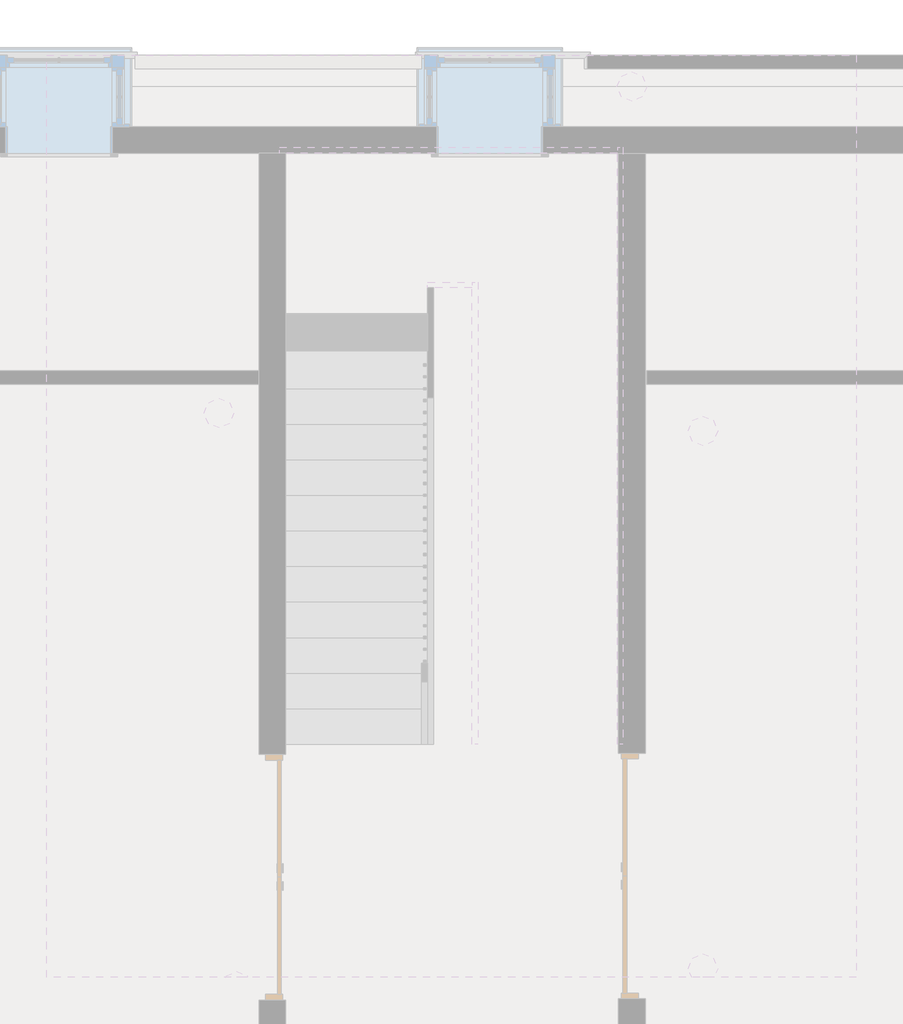
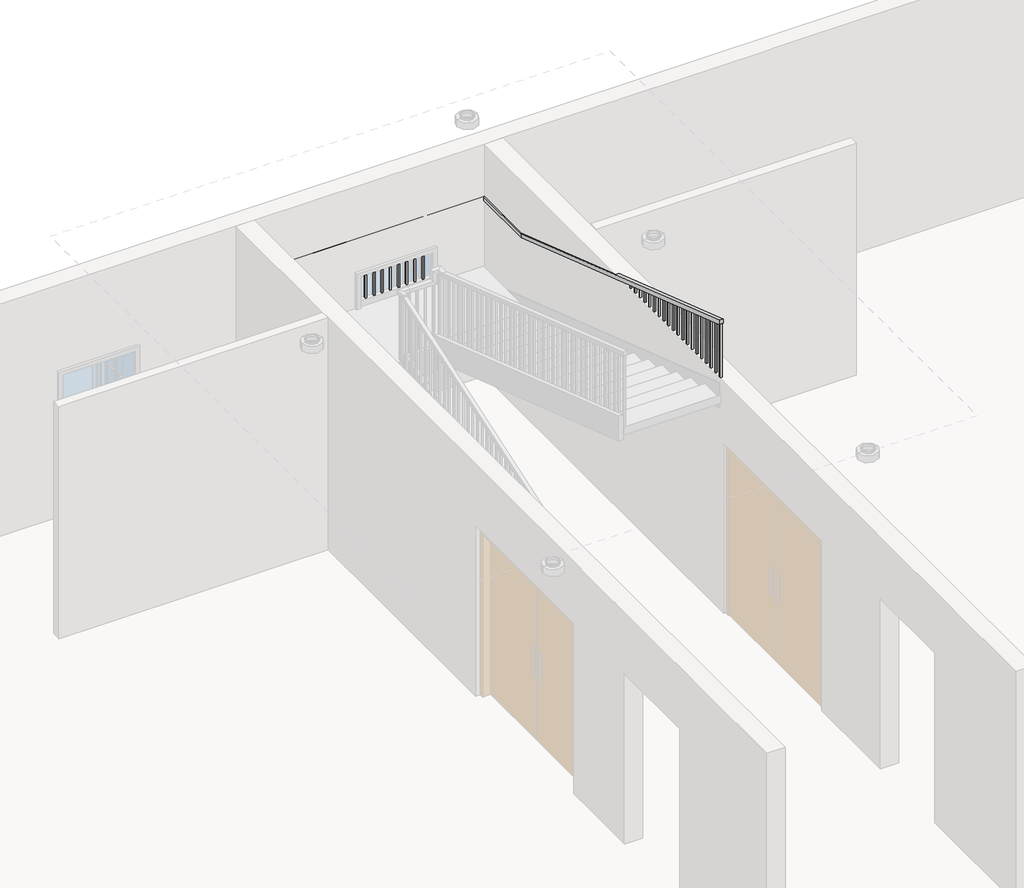
# One storey, part 5 of 7: 1 railing.
"""IFC4 building model written with IfcOpenShell, lengths in millimetres."""

from ifc_helpers import new_model, si_unit, frame, origin, place, context, project, spatial, polyline, outline, extrude, faceted_brep, element, save

model = new_model("IFC4")

# Units and contexts
model_context = context("Model", 3, world=origin())
ifc_project = project(units=[si_unit("LENGTHUNIT", "METRE", prefix="MILLI")], contexts=[model_context])

# Site, building, storey
site = spatial("IfcSite", under=ifc_project)
building = spatial("IfcBuilding", under=site)
storey = spatial("IfcBuildingStorey", under=building, Elevation=3200.4)

# Railing
placement = place(None, origin())
element("IfcRailing", 1, ObjectType="Handrail - Rectangular", at=placement, inside=storey, context=model_context, shape_type="SolidModel", body=[
    faceted_brep([(-1899.5987998, 2564.5067329, 4218.2142857), (-1899.5987998, 2564.5067329, 4164.5699957), (-1848.7987998, 2564.5067329, 4164.5699957), (-1848.7987998, 2564.5067329, 4218.2142857), (-1899.5987998, 6526.9067329, 5562.6), (-1899.5987998, 6535.2899033, 5511.8), (-1848.7987998, 6535.2899033, 5511.8), (-1848.7987998, 6526.9067329, 5562.6), (-1899.5987998, 7682.6067329, 5511.8), (-1899.5987998, 7682.6067329, 5562.6), (1046.8012002, 7682.6067329, 5562.6), (1046.8012002, 7682.6067329, 5511.8), (-1848.7987998, 7631.8067329, 5511.8), (996.0012002, 7631.8067329, 5511.8), (-1848.7987998, 7631.8067329, 5562.6), (996.0012002, 7631.8067329, 5562.6), (1046.8012002, 6831.7067329, 5562.6), (1046.8012002, 6823.3235624, 5511.8), (996.0012002, 6823.3235624, 5511.8), (996.0012002, 6831.7067329, 5562.6), (1046.8012002, 2564.5067329, 7010.4), (996.0012002, 2564.5067329, 7010.4), (996.0012002, 2564.5067329, 6956.75571), (1046.8012002, 2564.5067329, 6956.75571)], [[[0, 1, 2, 3]], [[1, 0, 4, 5]], [[2, 1, 5, 6]], [[3, 2, 6, 7]], [[0, 3, 7, 4]], [[8, 9, 10, 11]], [[12, 8, 11, 13]], [[14, 12, 13, 15]], [[9, 14, 15, 10]], [[11, 10, 16, 17]], [[13, 11, 17, 18]], [[15, 13, 18, 19]], [[10, 15, 19, 16]], [[5, 4, 9, 8]], [[6, 5, 8, 12]], [[7, 6, 12, 14]], [[4, 7, 14, 9]], [[20, 21, 22, 23]], [[17, 16, 20, 23]], [[18, 17, 23, 22]], [[19, 18, 22, 21]], [[16, 19, 21, 20]]]),
    extrude(outline(polyline([(2586.7317329, 6949.215085), (2586.7317329, 6178.2831452), (2567.6817329, 6184.7465381), (2567.6817329, 6955.6784779), (2586.7317329, 6949.215085)])), frame((1011.8762002, 0.0, 0.0), z_axis=(1.0, 0.0, 0.0), x_axis=(0.0, 1.0, 0.0)), (0.0, 0.0, 1.0), 19.05),
    extrude(outline(polyline([(2688.3317329, 6914.7436565), (2688.3317329, 6143.8117167), (2669.2817329, 6150.2751095), (2669.2817329, 6921.2070493), (2688.3317329, 6914.7436565)])), frame((1011.8762002, 0.0, 0.0), z_axis=(1.0, 0.0, 0.0), x_axis=(0.0, 1.0, 0.0)), (0.0, 0.0, 1.0), 19.05),
    extrude(outline(polyline([(2789.9317329, 6880.2722279), (2789.9317329, 6109.3402881), (2770.8817329, 6115.803681), (2770.8817329, 6886.7356207), (2789.9317329, 6880.2722279)])), frame((1011.8762002, 0.0, 0.0), z_axis=(1.0, 0.0, 0.0), x_axis=(0.0, 1.0, 0.0)), (0.0, 0.0, 1.0), 19.05),
    extrude(outline(polyline([(2891.5317329, 6845.8007993), (2891.5317329, 6074.8688595), (2872.4817329, 6081.3322524), (2872.4817329, 6852.2641922), (2891.5317329, 6845.8007993)])), frame((1011.8762002, 0.0, 0.0), z_axis=(1.0, 0.0, 0.0), x_axis=(0.0, 1.0, 0.0)), (0.0, 0.0, 1.0), 19.05),
    extrude(outline(polyline([(2993.1317329, 6811.3293707), (2993.1317329, 6040.397431), (2974.0817329, 6046.8608238), (2974.0817329, 6817.7927636), (2993.1317329, 6811.3293707)])), frame((1011.8762002, 0.0, 0.0), z_axis=(1.0, 0.0, 0.0), x_axis=(0.0, 1.0, 0.0)), (0.0, 0.0, 1.0), 19.05),
    extrude(outline(polyline([(3094.7317329, 6776.8579422), (3094.7317329, 6005.9260024), (3075.6817329, 6012.3893952), (3075.6817329, 6783.321335), (3094.7317329, 6776.8579422)])), frame((1011.8762002, 0.0, 0.0), z_axis=(1.0, 0.0, 0.0), x_axis=(0.0, 1.0, 0.0)), (0.0, 0.0, 1.0), 19.05),
    extrude(outline(polyline([(3196.3317329, 6742.3865136), (3196.3317329, 5971.4545738), (3177.2817329, 5977.9179667), (3177.2817329, 6748.8499065), (3196.3317329, 6742.3865136)])), frame((1011.8762002, 0.0, 0.0), z_axis=(1.0, 0.0, 0.0), x_axis=(0.0, 1.0, 0.0)), (0.0, 0.0, 1.0), 19.05),
    extrude(outline(polyline([(3297.9317329, 6707.915085), (3297.9317329, 5936.9831452), (3278.8817329, 5943.4465381), (3278.8817329, 6714.3784779), (3297.9317329, 6707.915085)])), frame((1011.8762002, 0.0, 0.0), z_axis=(1.0, 0.0, 0.0), x_axis=(0.0, 1.0, 0.0)), (0.0, 0.0, 1.0), 19.05),
    extrude(outline(polyline([(3399.5317329, 6673.4436565), (3399.5317329, 5902.5117167), (3380.4817329, 5908.9751095), (3380.4817329, 6679.9070493), (3399.5317329, 6673.4436565)])), frame((1011.8762002, 0.0, 0.0), z_axis=(1.0, 0.0, 0.0), x_axis=(0.0, 1.0, 0.0)), (0.0, 0.0, 1.0), 19.05),
    extrude(outline(polyline([(3501.1317329, 6638.9722279), (3501.1317329, 5868.0402881), (3482.0817329, 5874.503681), (3482.0817329, 6645.4356207), (3501.1317329, 6638.9722279)])), frame((1011.8762002, 0.0, 0.0), z_axis=(1.0, 0.0, 0.0), x_axis=(0.0, 1.0, 0.0)), (0.0, 0.0, 1.0), 19.05),
    extrude(outline(polyline([(3602.7317329, 6604.5007993), (3602.7317329, 5833.5688595), (3583.6817329, 5840.0322524), (3583.6817329, 6610.9641922), (3602.7317329, 6604.5007993)])), frame((1011.8762002, 0.0, 0.0), z_axis=(1.0, 0.0, 0.0), x_axis=(0.0, 1.0, 0.0)), (0.0, 0.0, 1.0), 19.05),
    extrude(outline(polyline([(3704.3317329, 6570.0293707), (3704.3317329, 5799.097431), (3685.2817329, 5805.5608238), (3685.2817329, 6576.4927636), (3704.3317329, 6570.0293707)])), frame((1011.8762002, 0.0, 0.0), z_axis=(1.0, 0.0, 0.0), x_axis=(0.0, 1.0, 0.0)), (0.0, 0.0, 1.0), 19.05),
    extrude(outline(polyline([(3805.9317329, 6535.5579422), (3805.9317329, 5764.6260024), (3786.8817329, 5771.0893952), (3786.8817329, 6542.021335), (3805.9317329, 6535.5579422)])), frame((1011.8762002, 0.0, 0.0), z_axis=(1.0, 0.0, 0.0), x_axis=(0.0, 1.0, 0.0)), (0.0, 0.0, 1.0), 19.05),
    extrude(outline(polyline([(3907.5317329, 6501.0865136), (3907.5317329, 5730.1545738), (3888.4817329, 5736.6179667), (3888.4817329, 6507.5499065), (3907.5317329, 6501.0865136)])), frame((1011.8762002, 0.0, 0.0), z_axis=(1.0, 0.0, 0.0), x_axis=(0.0, 1.0, 0.0)), (0.0, 0.0, 1.0), 19.05),
    extrude(outline(polyline([(4009.1317329, 6466.615085), (4009.1317329, 5695.6831452), (3990.0817329, 5702.1465381), (3990.0817329, 6473.0784779), (4009.1317329, 6466.615085)])), frame((1011.8762002, 0.0, 0.0), z_axis=(1.0, 0.0, 0.0), x_axis=(0.0, 1.0, 0.0)), (0.0, 0.0, 1.0), 19.05),
    extrude(outline(polyline([(4110.7317329, 6432.1436565), (4110.7317329, 5661.2117167), (4091.6817329, 5667.6751095), (4091.6817329, 6438.6070493), (4110.7317329, 6432.1436565)])), frame((1011.8762002, 0.0, 0.0), z_axis=(1.0, 0.0, 0.0), x_axis=(0.0, 1.0, 0.0)), (0.0, 0.0, 1.0), 19.05),
    extrude(outline(polyline([(4212.3317329, 6397.6722279), (4212.3317329, 5626.7402881), (4193.2817329, 5633.203681), (4193.2817329, 6404.1356207), (4212.3317329, 6397.6722279)])), frame((1011.8762002, 0.0, 0.0), z_axis=(1.0, 0.0, 0.0), x_axis=(0.0, 1.0, 0.0)), (0.0, 0.0, 1.0), 19.05),
    extrude(outline(polyline([(4313.9317329, 6363.2007993), (4313.9317329, 5592.2688595), (4294.8817329, 5598.7322524), (4294.8817329, 6369.6641922), (4313.9317329, 6363.2007993)])), frame((1011.8762002, 0.0, 0.0), z_axis=(1.0, 0.0, 0.0), x_axis=(0.0, 1.0, 0.0)), (0.0, 0.0, 1.0), 19.05),
    extrude(outline(polyline([(4415.5317329, 6328.7293707), (4415.5317329, 5557.797431), (4396.4817329, 5564.2608238), (4396.4817329, 6335.1927636), (4415.5317329, 6328.7293707)])), frame((1011.8762002, 0.0, 0.0), z_axis=(1.0, 0.0, 0.0), x_axis=(0.0, 1.0, 0.0)), (0.0, 0.0, 1.0), 19.05),
    extrude(outline(polyline([(4517.1317329, 6294.2579422), (4517.1317329, 5523.3260024), (4498.0817329, 5529.7893952), (4498.0817329, 6300.721335), (4517.1317329, 6294.2579422)])), frame((1011.8762002, 0.0, 0.0), z_axis=(1.0, 0.0, 0.0), x_axis=(0.0, 1.0, 0.0)), (0.0, 0.0, 1.0), 19.05),
    extrude(outline(polyline([(4618.7317329, 6259.7865136), (4618.7317329, 5488.8545738), (4599.6817329, 5495.3179667), (4599.6817329, 6266.2499065), (4618.7317329, 6259.7865136)])), frame((1011.8762002, 0.0, 0.0), z_axis=(1.0, 0.0, 0.0), x_axis=(0.0, 1.0, 0.0)), (0.0, 0.0, 1.0), 19.05),
    extrude(outline(polyline([(4720.3317329, 6225.315085), (4720.3317329, 5454.3831452), (4701.2817329, 5460.8465381), (4701.2817329, 6231.7784779), (4720.3317329, 6225.315085)])), frame((1011.8762002, 0.0, 0.0), z_axis=(1.0, 0.0, 0.0), x_axis=(0.0, 1.0, 0.0)), (0.0, 0.0, 1.0), 19.05),
    extrude(outline(polyline([(4821.9317329, 6190.8436565), (4821.9317329, 5419.9117167), (4802.8817329, 5426.3751095), (4802.8817329, 6197.3070493), (4821.9317329, 6190.8436565)])), frame((1011.8762002, 0.0, 0.0), z_axis=(1.0, 0.0, 0.0), x_axis=(0.0, 1.0, 0.0)), (0.0, 0.0, 1.0), 19.05),
    extrude(outline(polyline([(4923.5317329, 6156.3722279), (4923.5317329, 5385.4402881), (4904.4817329, 5391.903681), (4904.4817329, 6162.8356207), (4923.5317329, 6156.3722279)])), frame((1011.8762002, 0.0, 0.0), z_axis=(1.0, 0.0, 0.0), x_axis=(0.0, 1.0, 0.0)), (0.0, 0.0, 1.0), 19.05),
    extrude(outline(polyline([(5025.1317329, 6121.9007993), (5025.1317329, 5350.9688595), (5006.0817329, 5357.4322524), (5006.0817329, 6128.3641922), (5025.1317329, 6121.9007993)])), frame((1011.8762002, 0.0, 0.0), z_axis=(1.0, 0.0, 0.0), x_axis=(0.0, 1.0, 0.0)), (0.0, 0.0, 1.0), 19.05),
    extrude(outline(polyline([(5126.7317329, 6087.4293707), (5126.7317329, 5316.497431), (5107.6817329, 5322.9608238), (5107.6817329, 6093.8927636), (5126.7317329, 6087.4293707)])), frame((1011.8762002, 0.0, 0.0), z_axis=(1.0, 0.0, 0.0), x_axis=(0.0, 1.0, 0.0)), (0.0, 0.0, 1.0), 19.05),
    extrude(outline(polyline([(5228.3317329, 6052.9579422), (5228.3317329, 5282.0260024), (5209.2817329, 5288.4893952), (5209.2817329, 6059.421335), (5228.3317329, 6052.9579422)])), frame((1011.8762002, 0.0, 0.0), z_axis=(1.0, 0.0, 0.0), x_axis=(0.0, 1.0, 0.0)), (0.0, 0.0, 1.0), 19.05),
    extrude(outline(polyline([(5329.9317329, 6018.4865136), (5329.9317329, 5247.5545738), (5310.8817329, 5254.0179667), (5310.8817329, 6024.9499065), (5329.9317329, 6018.4865136)])), frame((1011.8762002, 0.0, 0.0), z_axis=(1.0, 0.0, 0.0), x_axis=(0.0, 1.0, 0.0)), (0.0, 0.0, 1.0), 19.05),
    extrude(outline(polyline([(5431.5317329, 5984.015085), (5431.5317329, 5213.0831452), (5412.4817329, 5219.5465381), (5412.4817329, 5990.4784779), (5431.5317329, 5984.015085)])), frame((1011.8762002, 0.0, 0.0), z_axis=(1.0, 0.0, 0.0), x_axis=(0.0, 1.0, 0.0)), (0.0, 0.0, 1.0), 19.05),
    extrude(outline(polyline([(5533.1317329, 5949.5436565), (5533.1317329, 5178.6117167), (5514.0817329, 5185.0751095), (5514.0817329, 5956.0070493), (5533.1317329, 5949.5436565)])), frame((1011.8762002, 0.0, 0.0), z_axis=(1.0, 0.0, 0.0), x_axis=(0.0, 1.0, 0.0)), (0.0, 0.0, 1.0), 19.05),
    extrude(outline(polyline([(5634.7317329, 5915.0722279), (5634.7317329, 5144.1402881), (5615.6817329, 5150.603681), (5615.6817329, 5921.5356207), (5634.7317329, 5915.0722279)])), frame((1011.8762002, 0.0, 0.0), z_axis=(1.0, 0.0, 0.0), x_axis=(0.0, 1.0, 0.0)), (0.0, 0.0, 1.0), 19.05),
    extrude(outline(polyline([(5736.3317329, 5880.6007993), (5736.3317329, 5109.6688595), (5717.2817329, 5116.1322524), (5717.2817329, 5887.0641922), (5736.3317329, 5880.6007993)])), frame((1011.8762002, 0.0, 0.0), z_axis=(1.0, 0.0, 0.0), x_axis=(0.0, 1.0, 0.0)), (0.0, 0.0, 1.0), 19.05),
    extrude(outline(polyline([(5837.9317329, 5846.1293707), (5837.9317329, 5075.197431), (5818.8817329, 5081.6608238), (5818.8817329, 5852.5927636), (5837.9317329, 5846.1293707)])), frame((1011.8762002, 0.0, 0.0), z_axis=(1.0, 0.0, 0.0), x_axis=(0.0, 1.0, 0.0)), (0.0, 0.0, 1.0), 19.05),
    extrude(outline(polyline([(5939.5317329, 5811.6579422), (5939.5317329, 5040.7260024), (5920.4817329, 5047.1893952), (5920.4817329, 5818.121335), (5939.5317329, 5811.6579422)])), frame((1011.8762002, 0.0, 0.0), z_axis=(1.0, 0.0, 0.0), x_axis=(0.0, 1.0, 0.0)), (0.0, 0.0, 1.0), 19.05),
    extrude(outline(polyline([(6041.1317329, 5777.1865136), (6041.1317329, 5006.2545738), (6022.0817329, 5012.7179667), (6022.0817329, 5783.6499065), (6041.1317329, 5777.1865136)])), frame((1011.8762002, 0.0, 0.0), z_axis=(1.0, 0.0, 0.0), x_axis=(0.0, 1.0, 0.0)), (0.0, 0.0, 1.0), 19.05),
    extrude(outline(polyline([(6142.7317329, 5742.715085), (6142.7317329, 4971.7831452), (6123.6817329, 4978.2465381), (6123.6817329, 5749.1784779), (6142.7317329, 5742.715085)])), frame((1011.8762002, 0.0, 0.0), z_axis=(1.0, 0.0, 0.0), x_axis=(0.0, 1.0, 0.0)), (0.0, 0.0, 1.0), 19.05),
    extrude(outline(polyline([(6244.3317329, 5708.2436565), (6244.3317329, 4937.3117167), (6225.2817329, 4943.7751095), (6225.2817329, 5714.7070493), (6244.3317329, 5708.2436565)])), frame((1011.8762002, 0.0, 0.0), z_axis=(1.0, 0.0, 0.0), x_axis=(0.0, 1.0, 0.0)), (0.0, 0.0, 1.0), 19.05),
    extrude(outline(polyline([(6345.9317329, 5673.7722279), (6345.9317329, 4902.8402881), (6326.8817329, 4909.303681), (6326.8817329, 5680.2356207), (6345.9317329, 5673.7722279)])), frame((1011.8762002, 0.0, 0.0), z_axis=(1.0, 0.0, 0.0), x_axis=(0.0, 1.0, 0.0)), (0.0, 0.0, 1.0), 19.05),
    extrude(outline(polyline([(6447.5317329, 5639.3007993), (6447.5317329, 4868.3688595), (6428.4817329, 4874.8322524), (6428.4817329, 5645.7641922), (6447.5317329, 5639.3007993)])), frame((1011.8762002, 0.0, 0.0), z_axis=(1.0, 0.0, 0.0), x_axis=(0.0, 1.0, 0.0)), (0.0, 0.0, 1.0), 19.05),
    extrude(outline(polyline([(6549.1317329, 5604.8293707), (6549.1317329, 4833.897431), (6530.0817329, 4840.3608238), (6530.0817329, 5611.2927636), (6549.1317329, 5604.8293707)])), frame((1011.8762002, 0.0, 0.0), z_axis=(1.0, 0.0, 0.0), x_axis=(0.0, 1.0, 0.0)), (0.0, 0.0, 1.0), 19.05),
    extrude(outline(polyline([(6650.7317329, 5570.3579422), (6650.7317329, 4799.4260024), (6631.6817329, 4805.8893952), (6631.6817329, 5576.821335), (6650.7317329, 5570.3579422)])), frame((1011.8762002, 0.0, 0.0), z_axis=(1.0, 0.0, 0.0), x_axis=(0.0, 1.0, 0.0)), (0.0, 0.0, 1.0), 19.05),
    extrude(outline(polyline([(6752.3317329, 5535.8865136), (6752.3317329, 4764.9545738), (6733.2817329, 4771.4179667), (6733.2817329, 5542.3499065), (6752.3317329, 5535.8865136)])), frame((1011.8762002, 0.0, 0.0), z_axis=(1.0, 0.0, 0.0), x_axis=(0.0, 1.0, 0.0)), (0.0, 0.0, 1.0), 19.05),
    extrude(outline(polyline([(6853.9317329, 5511.8), (6853.9317329, 4730.4831452), (6834.8817329, 4736.9465381), (6834.8817329, 5511.8), (6853.9317329, 5511.8)])), frame((1011.8762002, 0.0, 0.0), z_axis=(1.0, 0.0, 0.0), x_axis=(0.0, 1.0, 0.0)), (0.0, 0.0, 1.0), 19.05),
    extrude(outline(polyline([(6955.5317329, 5511.8), (6955.5317329, 4696.0117167), (6936.4817329, 4702.4751095), (6936.4817329, 5511.8), (6955.5317329, 5511.8)])), frame((1011.8762002, 0.0, 0.0), z_axis=(1.0, 0.0, 0.0), x_axis=(0.0, 1.0, 0.0)), (0.0, 0.0, 1.0), 19.05),
    extrude(outline(polyline([(7057.1317329, 5511.8), (7057.1317329, 4661.5402881), (7038.0817329, 4668.003681), (7038.0817329, 5511.8), (7057.1317329, 5511.8)])), frame((1011.8762002, 0.0, 0.0), z_axis=(1.0, 0.0, 0.0), x_axis=(0.0, 1.0, 0.0)), (0.0, 0.0, 1.0), 19.05),
    extrude(outline(polyline([(7158.7317329, 5511.8), (7158.7317329, 4627.0688595), (7139.6817329, 4633.5322524), (7139.6817329, 5511.8), (7158.7317329, 5511.8)])), frame((1011.8762002, 0.0, 0.0), z_axis=(1.0, 0.0, 0.0), x_axis=(0.0, 1.0, 0.0)), (0.0, 0.0, 1.0), 19.05),
    extrude(outline(polyline([(7260.3317329, 5511.8), (7260.3317329, 4592.597431), (7241.2817329, 4599.0608238), (7241.2817329, 5511.8), (7260.3317329, 5511.8)])), frame((1011.8762002, 0.0, 0.0), z_axis=(1.0, 0.0, 0.0), x_axis=(0.0, 1.0, 0.0)), (0.0, 0.0, 1.0), 19.05),
    extrude(outline(polyline([(7361.9317329, 5511.8), (7361.9317329, 4558.1260024), (7342.8817329, 4564.5893952), (7342.8817329, 5511.8), (7361.9317329, 5511.8)])), frame((1011.8762002, 0.0, 0.0), z_axis=(1.0, 0.0, 0.0), x_axis=(0.0, 1.0, 0.0)), (0.0, 0.0, 1.0), 19.05),
    extrude(outline(polyline([(7463.5317329, 5511.8), (7463.5317329, 4523.6545738), (7444.4817329, 4530.1179667), (7444.4817329, 5511.8), (7463.5317329, 5511.8)])), frame((1011.8762002, 0.0, 0.0), z_axis=(1.0, 0.0, 0.0), x_axis=(0.0, 1.0, 0.0)), (0.0, 0.0, 1.0), 19.05),
    extrude(outline(polyline([(7565.1317329, 5511.8), (7565.1317329, 4489.1831452), (7546.0817329, 4495.6465381), (7546.0817329, 5511.8), (7565.1317329, 5511.8)])), frame((1011.8762002, 0.0, 0.0), z_axis=(1.0, 0.0, 0.0), x_axis=(0.0, 1.0, 0.0)), (0.0, 0.0, 1.0), 19.05),
    extrude(outline(polyline([(961.0762002, 7666.7317329), (980.1262002, 7666.7317329), (980.1262002, 7647.6817329), (961.0762002, 7647.6817329), (961.0762002, 7666.7317329)])), frame((0.0, 0.0, 4724.4), z_axis=(0.0, 0.0, 1.0), x_axis=(1.0, 0.0, 0.0)), (0.0, 0.0, 1.0), 787.4),
    extrude(outline(polyline([(859.4762002, 7666.7317329), (878.5262002, 7666.7317329), (878.5262002, 7647.6817329), (859.4762002, 7647.6817329), (859.4762002, 7666.7317329)])), frame((0.0, 0.0, 4724.4), z_axis=(0.0, 0.0, 1.0), x_axis=(1.0, 0.0, 0.0)), (0.0, 0.0, 1.0), 787.4),
    extrude(outline(polyline([(757.8762002, 7666.7317329), (776.9262002, 7666.7317329), (776.9262002, 7647.6817329), (757.8762002, 7647.6817329), (757.8762002, 7666.7317329)])), frame((0.0, 0.0, 4724.4), z_axis=(0.0, 0.0, 1.0), x_axis=(1.0, 0.0, 0.0)), (0.0, 0.0, 1.0), 787.4),
    extrude(outline(polyline([(656.2762002, 7666.7317329), (675.3262002, 7666.7317329), (675.3262002, 7647.6817329), (656.2762002, 7647.6817329), (656.2762002, 7666.7317329)])), frame((0.0, 0.0, 4724.4), z_axis=(0.0, 0.0, 1.0), x_axis=(1.0, 0.0, 0.0)), (0.0, 0.0, 1.0), 787.4),
    extrude(outline(polyline([(554.6762002, 7666.7317329), (573.7262002, 7666.7317329), (573.7262002, 7647.6817329), (554.6762002, 7647.6817329), (554.6762002, 7666.7317329)])), frame((0.0, 0.0, 4724.4), z_axis=(0.0, 0.0, 1.0), x_axis=(1.0, 0.0, 0.0)), (0.0, 0.0, 1.0), 787.4),
    extrude(outline(polyline([(453.0762002, 7666.7317329), (472.1262002, 7666.7317329), (472.1262002, 7647.6817329), (453.0762002, 7647.6817329), (453.0762002, 7666.7317329)])), frame((0.0, 0.0, 4724.4), z_axis=(0.0, 0.0, 1.0), x_axis=(1.0, 0.0, 0.0)), (0.0, 0.0, 1.0), 787.4),
    extrude(outline(polyline([(351.4762002, 7666.7317329), (370.5262002, 7666.7317329), (370.5262002, 7647.6817329), (351.4762002, 7647.6817329), (351.4762002, 7666.7317329)])), frame((0.0, 0.0, 4724.4), z_axis=(0.0, 0.0, 1.0), x_axis=(1.0, 0.0, 0.0)), (0.0, 0.0, 1.0), 787.4),
    extrude(outline(polyline([(249.8762002, 7666.7317329), (268.9262002, 7666.7317329), (268.9262002, 7647.6817329), (249.8762002, 7647.6817329), (249.8762002, 7666.7317329)])), frame((0.0, 0.0, 4724.4), z_axis=(0.0, 0.0, 1.0), x_axis=(1.0, 0.0, 0.0)), (0.0, 0.0, 1.0), 787.4),
    extrude(outline(polyline([(148.2762002, 7666.7317329), (167.3262002, 7666.7317329), (167.3262002, 7647.6817329), (148.2762002, 7647.6817329), (148.2762002, 7666.7317329)])), frame((0.0, 0.0, 4724.4), z_axis=(0.0, 0.0, 1.0), x_axis=(1.0, 0.0, 0.0)), (0.0, 0.0, 1.0), 787.4),
    extrude(outline(polyline([(46.6762002, 7666.7317329), (65.7262002, 7666.7317329), (65.7262002, 7647.6817329), (46.6762002, 7647.6817329), (46.6762002, 7666.7317329)])), frame((0.0, 0.0, 4724.4), z_axis=(0.0, 0.0, 1.0), x_axis=(1.0, 0.0, 0.0)), (0.0, 0.0, 1.0), 787.4),
    extrude(outline(polyline([(-54.9237998, 7666.7317329), (-35.8737998, 7666.7317329), (-35.8737998, 7647.6817329), (-54.9237998, 7647.6817329), (-54.9237998, 7666.7317329)])), frame((0.0, 0.0, 4724.4), z_axis=(0.0, 0.0, 1.0), x_axis=(1.0, 0.0, 0.0)), (0.0, 0.0, 1.0), 787.4),
    extrude(outline(polyline([(-156.5237998, 7666.7317329), (-137.4737998, 7666.7317329), (-137.4737998, 7647.6817329), (-156.5237998, 7647.6817329), (-156.5237998, 7666.7317329)])), frame((0.0, 0.0, 4724.4), z_axis=(0.0, 0.0, 1.0), x_axis=(1.0, 0.0, 0.0)), (0.0, 0.0, 1.0), 787.4),
    extrude(outline(polyline([(-258.1237998, 7666.7317329), (-239.0737998, 7666.7317329), (-239.0737998, 7647.6817329), (-258.1237998, 7647.6817329), (-258.1237998, 7666.7317329)])), frame((0.0, 0.0, 4724.4), z_axis=(0.0, 0.0, 1.0), x_axis=(1.0, 0.0, 0.0)), (0.0, 0.0, 1.0), 787.4),
    extrude(outline(polyline([(-359.7237998, 7666.7317329), (-340.6737998, 7666.7317329), (-340.6737998, 7647.6817329), (-359.7237998, 7647.6817329), (-359.7237998, 7666.7317329)])), frame((0.0, 0.0, 4724.4), z_axis=(0.0, 0.0, 1.0), x_axis=(1.0, 0.0, 0.0)), (0.0, 0.0, 1.0), 787.4),
    extrude(outline(polyline([(-461.3237998, 7666.7317329), (-442.2737998, 7666.7317329), (-442.2737998, 7647.6817329), (-461.3237998, 7647.6817329), (-461.3237998, 7666.7317329)])), frame((0.0, 0.0, 4724.4), z_axis=(0.0, 0.0, 1.0), x_axis=(1.0, 0.0, 0.0)), (0.0, 0.0, 1.0), 787.4),
    extrude(outline(polyline([(-562.9237998, 7666.7317329), (-543.8737998, 7666.7317329), (-543.8737998, 7647.6817329), (-562.9237998, 7647.6817329), (-562.9237998, 7666.7317329)])), frame((0.0, 0.0, 4724.4), z_axis=(0.0, 0.0, 1.0), x_axis=(1.0, 0.0, 0.0)), (0.0, 0.0, 1.0), 787.4),
    extrude(outline(polyline([(-664.5237998, 7666.7317329), (-645.4737998, 7666.7317329), (-645.4737998, 7647.6817329), (-664.5237998, 7647.6817329), (-664.5237998, 7666.7317329)])), frame((0.0, 0.0, 4724.4), z_axis=(0.0, 0.0, 1.0), x_axis=(1.0, 0.0, 0.0)), (0.0, 0.0, 1.0), 787.4),
    extrude(outline(polyline([(-766.1237998, 7666.7317329), (-747.0737998, 7666.7317329), (-747.0737998, 7647.6817329), (-766.1237998, 7647.6817329), (-766.1237998, 7666.7317329)])), frame((0.0, 0.0, 4724.4), z_axis=(0.0, 0.0, 1.0), x_axis=(1.0, 0.0, 0.0)), (0.0, 0.0, 1.0), 787.4),
    extrude(outline(polyline([(-867.7237998, 7666.7317329), (-848.6737998, 7666.7317329), (-848.6737998, 7647.6817329), (-867.7237998, 7647.6817329), (-867.7237998, 7666.7317329)])), frame((0.0, 0.0, 4724.4), z_axis=(0.0, 0.0, 1.0), x_axis=(1.0, 0.0, 0.0)), (0.0, 0.0, 1.0), 787.4),
    extrude(outline(polyline([(-969.3237998, 7666.7317329), (-950.2737998, 7666.7317329), (-950.2737998, 7647.6817329), (-969.3237998, 7647.6817329), (-969.3237998, 7666.7317329)])), frame((0.0, 0.0, 4724.4), z_axis=(0.0, 0.0, 1.0), x_axis=(1.0, 0.0, 0.0)), (0.0, 0.0, 1.0), 787.4),
    extrude(outline(polyline([(-1070.9237998, 7666.7317329), (-1051.8737998, 7666.7317329), (-1051.8737998, 7647.6817329), (-1070.9237998, 7647.6817329), (-1070.9237998, 7666.7317329)])), frame((0.0, 0.0, 4724.4), z_axis=(0.0, 0.0, 1.0), x_axis=(1.0, 0.0, 0.0)), (0.0, 0.0, 1.0), 787.4),
    extrude(outline(polyline([(-1172.5237998, 7666.7317329), (-1153.4737998, 7666.7317329), (-1153.4737998, 7647.6817329), (-1172.5237998, 7647.6817329), (-1172.5237998, 7666.7317329)])), frame((0.0, 0.0, 4724.4), z_axis=(0.0, 0.0, 1.0), x_axis=(1.0, 0.0, 0.0)), (0.0, 0.0, 1.0), 787.4),
    extrude(outline(polyline([(-1274.1237998, 7666.7317329), (-1255.0737998, 7666.7317329), (-1255.0737998, 7647.6817329), (-1274.1237998, 7647.6817329), (-1274.1237998, 7666.7317329)])), frame((0.0, 0.0, 4724.4), z_axis=(0.0, 0.0, 1.0), x_axis=(1.0, 0.0, 0.0)), (0.0, 0.0, 1.0), 787.4),
    extrude(outline(polyline([(-1375.7237998, 7666.7317329), (-1356.6737998, 7666.7317329), (-1356.6737998, 7647.6817329), (-1375.7237998, 7647.6817329), (-1375.7237998, 7666.7317329)])), frame((0.0, 0.0, 4724.4), z_axis=(0.0, 0.0, 1.0), x_axis=(1.0, 0.0, 0.0)), (0.0, 0.0, 1.0), 787.4),
    extrude(outline(polyline([(-1477.3237998, 7666.7317329), (-1458.2737998, 7666.7317329), (-1458.2737998, 7647.6817329), (-1477.3237998, 7647.6817329), (-1477.3237998, 7666.7317329)])), frame((0.0, 0.0, 4724.4), z_axis=(0.0, 0.0, 1.0), x_axis=(1.0, 0.0, 0.0)), (0.0, 0.0, 1.0), 787.4),
    extrude(outline(polyline([(-1578.9237998, 7666.7317329), (-1559.8737998, 7666.7317329), (-1559.8737998, 7647.6817329), (-1578.9237998, 7647.6817329), (-1578.9237998, 7666.7317329)])), frame((0.0, 0.0, 4724.4), z_axis=(0.0, 0.0, 1.0), x_axis=(1.0, 0.0, 0.0)), (0.0, 0.0, 1.0), 787.4),
    extrude(outline(polyline([(-1680.5237998, 7666.7317329), (-1661.4737998, 7666.7317329), (-1661.4737998, 7647.6817329), (-1680.5237998, 7647.6817329), (-1680.5237998, 7666.7317329)])), frame((0.0, 0.0, 4724.4), z_axis=(0.0, 0.0, 1.0), x_axis=(1.0, 0.0, 0.0)), (0.0, 0.0, 1.0), 787.4),
    extrude(outline(polyline([(-1782.1237998, 7666.7317329), (-1763.0737998, 7666.7317329), (-1763.0737998, 7647.6817329), (-1782.1237998, 7647.6817329), (-1782.1237998, 7666.7317329)])), frame((0.0, 0.0, 4724.4), z_axis=(0.0, 0.0, 1.0), x_axis=(1.0, 0.0, 0.0)), (0.0, 0.0, 1.0), 787.4),
    extrude(outline(polyline([(-1883.7237998, 7634.9817329), (-1883.7237998, 7654.0317329), (-1864.6737998, 7654.0317329), (-1864.6737998, 7634.9817329), (-1883.7237998, 7634.9817329)])), frame((0.0, 0.0, 5027.3857143), z_axis=(0.0, 0.0, 1.0), x_axis=(1.0, 0.0, 0.0)), (0.0, 0.0, 1.0), 484.4142857),
    extrude(outline(polyline([(-1883.7237998, 7533.3817329), (-1883.7237998, 7552.4317329), (-1864.6737998, 7552.4317329), (-1864.6737998, 7533.3817329), (-1883.7237998, 7533.3817329)])), frame((0.0, 0.0, 4992.9142857), z_axis=(0.0, 0.0, 1.0), x_axis=(1.0, 0.0, 0.0)), (0.0, 0.0, 1.0), 518.8857143),
    extrude(outline(polyline([(-1883.7237998, 7431.7817329), (-1883.7237998, 7450.8317329), (-1864.6737998, 7450.8317329), (-1864.6737998, 7431.7817329), (-1883.7237998, 7431.7817329)])), frame((0.0, 0.0, 4958.4428571), z_axis=(0.0, 0.0, 1.0), x_axis=(1.0, 0.0, 0.0)), (0.0, 0.0, 1.0), 553.3571429),
    extrude(outline(polyline([(-1883.7237998, 7330.1817329), (-1883.7237998, 7349.2317329), (-1864.6737998, 7349.2317329), (-1864.6737998, 7330.1817329), (-1883.7237998, 7330.1817329)])), frame((0.0, 0.0, 4923.9714286), z_axis=(0.0, 0.0, 1.0), x_axis=(1.0, 0.0, 0.0)), (0.0, 0.0, 1.0), 587.8285714),
    extrude(outline(polyline([(-1883.7237998, 7228.5817329), (-1883.7237998, 7247.6317329), (-1864.6737998, 7247.6317329), (-1864.6737998, 7228.5817329), (-1883.7237998, 7228.5817329)])), frame((0.0, 0.0, 4889.5), z_axis=(0.0, 0.0, 1.0), x_axis=(1.0, 0.0, 0.0)), (0.0, 0.0, 1.0), 622.3),
    extrude(outline(polyline([(-1883.7237998, 7126.9817329), (-1883.7237998, 7146.0317329), (-1864.6737998, 7146.0317329), (-1864.6737998, 7126.9817329), (-1883.7237998, 7126.9817329)])), frame((0.0, 0.0, 4855.0285714), z_axis=(0.0, 0.0, 1.0), x_axis=(1.0, 0.0, 0.0)), (0.0, 0.0, 1.0), 656.7714286),
    extrude(outline(polyline([(-1883.7237998, 7025.3817329), (-1883.7237998, 7044.4317329), (-1864.6737998, 7044.4317329), (-1864.6737998, 7025.3817329), (-1883.7237998, 7025.3817329)])), frame((0.0, 0.0, 4724.4), z_axis=(0.0, 0.0, 1.0), x_axis=(1.0, 0.0, 0.0)), (0.0, 0.0, 1.0), 787.4),
    extrude(outline(polyline([(-1883.7237998, 6923.7817329), (-1883.7237998, 6942.8317329), (-1864.6737998, 6942.8317329), (-1864.6737998, 6923.7817329), (-1883.7237998, 6923.7817329)])), frame((0.0, 0.0, 4724.4), z_axis=(0.0, 0.0, 1.0), x_axis=(1.0, 0.0, 0.0)), (0.0, 0.0, 1.0), 787.4),
    extrude(outline(polyline([(-1883.7237998, 6822.1817329), (-1883.7237998, 6841.2317329), (-1864.6737998, 6841.2317329), (-1864.6737998, 6822.1817329), (-1883.7237998, 6822.1817329)])), frame((0.0, 0.0, 4724.4), z_axis=(0.0, 0.0, 1.0), x_axis=(1.0, 0.0, 0.0)), (0.0, 0.0, 1.0), 787.4),
    extrude(outline(polyline([(-1883.7237998, 6720.5817329), (-1883.7237998, 6739.6317329), (-1864.6737998, 6739.6317329), (-1864.6737998, 6720.5817329), (-1883.7237998, 6720.5817329)])), frame((0.0, 0.0, 4724.4), z_axis=(0.0, 0.0, 1.0), x_axis=(1.0, 0.0, 0.0)), (0.0, 0.0, 1.0), 787.4),
    extrude(outline(polyline([(-1883.7237998, 6618.9817329), (-1883.7237998, 6638.0317329), (-1864.6737998, 6638.0317329), (-1864.6737998, 6618.9817329), (-1883.7237998, 6618.9817329)])), frame((0.0, 0.0, 4724.4), z_axis=(0.0, 0.0, 1.0), x_axis=(1.0, 0.0, 0.0)), (0.0, 0.0, 1.0), 787.4),
    extrude(outline(polyline([(6536.4317329, 5512.1874065), (6536.4317329, 4724.4), (6517.3817329, 4724.4), (6517.3817329, 5505.7240136), (6536.4317329, 5512.1874065)])), frame((-1883.7237998, 0.0, 0.0), z_axis=(1.0, 0.0, 0.0), x_axis=(0.0, 1.0, 0.0)), (0.0, 0.0, 1.0), 19.05),
    extrude(outline(polyline([(6434.8317329, 5477.7159779), (6434.8317329, 4706.7840381), (6415.7817329, 4700.3206452), (6415.7817329, 5471.252585), (6434.8317329, 5477.7159779)])), frame((-1883.7237998, 0.0, 0.0), z_axis=(1.0, 0.0, 0.0), x_axis=(0.0, 1.0, 0.0)), (0.0, 0.0, 1.0), 19.05),
    extrude(outline(polyline([(6333.2317329, 5443.2445493), (6333.2317329, 4672.3126095), (6314.1817329, 4665.8492167), (6314.1817329, 5436.7811565), (6333.2317329, 5443.2445493)])), frame((-1883.7237998, 0.0, 0.0), z_axis=(1.0, 0.0, 0.0), x_axis=(0.0, 1.0, 0.0)), (0.0, 0.0, 1.0), 19.05),
    extrude(outline(polyline([(6231.6317329, 5408.7731207), (6231.6317329, 4637.841181), (6212.5817329, 4631.3777881), (6212.5817329, 5402.3097279), (6231.6317329, 5408.7731207)])), frame((-1883.7237998, 0.0, 0.0), z_axis=(1.0, 0.0, 0.0), x_axis=(0.0, 1.0, 0.0)), (0.0, 0.0, 1.0), 19.05),
    extrude(outline(polyline([(6130.0317329, 5374.3016922), (6130.0317329, 4603.3697524), (6110.9817329, 4596.9063595), (6110.9817329, 5367.8382993), (6130.0317329, 5374.3016922)])), frame((-1883.7237998, 0.0, 0.0), z_axis=(1.0, 0.0, 0.0), x_axis=(0.0, 1.0, 0.0)), (0.0, 0.0, 1.0), 19.05),
    extrude(outline(polyline([(6028.4317329, 5339.8302636), (6028.4317329, 4568.8983238), (6009.3817329, 4562.434931), (6009.3817329, 5333.3668707), (6028.4317329, 5339.8302636)])), frame((-1883.7237998, 0.0, 0.0), z_axis=(1.0, 0.0, 0.0), x_axis=(0.0, 1.0, 0.0)), (0.0, 0.0, 1.0), 19.05),
    extrude(outline(polyline([(5926.8317329, 5305.358835), (5926.8317329, 4534.4268952), (5907.7817329, 4527.9635024), (5907.7817329, 5298.8954422), (5926.8317329, 5305.358835)])), frame((-1883.7237998, 0.0, 0.0), z_axis=(1.0, 0.0, 0.0), x_axis=(0.0, 1.0, 0.0)), (0.0, 0.0, 1.0), 19.05),
    extrude(outline(polyline([(5825.2317329, 5270.8874065), (5825.2317329, 4499.9554667), (5806.1817329, 4493.4920738), (5806.1817329, 5264.4240136), (5825.2317329, 5270.8874065)])), frame((-1883.7237998, 0.0, 0.0), z_axis=(1.0, 0.0, 0.0), x_axis=(0.0, 1.0, 0.0)), (0.0, 0.0, 1.0), 19.05),
    extrude(outline(polyline([(5723.6317329, 5236.4159779), (5723.6317329, 4465.4840381), (5704.5817329, 4459.0206452), (5704.5817329, 5229.952585), (5723.6317329, 5236.4159779)])), frame((-1883.7237998, 0.0, 0.0), z_axis=(1.0, 0.0, 0.0), x_axis=(0.0, 1.0, 0.0)), (0.0, 0.0, 1.0), 19.05),
    extrude(outline(polyline([(5622.0317329, 5201.9445493), (5622.0317329, 4431.0126095), (5602.9817329, 4424.5492167), (5602.9817329, 5195.4811565), (5622.0317329, 5201.9445493)])), frame((-1883.7237998, 0.0, 0.0), z_axis=(1.0, 0.0, 0.0), x_axis=(0.0, 1.0, 0.0)), (0.0, 0.0, 1.0), 19.05),
    extrude(outline(polyline([(5520.4317329, 5167.4731207), (5520.4317329, 4396.541181), (5501.3817329, 4390.0777881), (5501.3817329, 5161.0097279), (5520.4317329, 5167.4731207)])), frame((-1883.7237998, 0.0, 0.0), z_axis=(1.0, 0.0, 0.0), x_axis=(0.0, 1.0, 0.0)), (0.0, 0.0, 1.0), 19.05),
    extrude(outline(polyline([(5418.8317329, 5133.0016922), (5418.8317329, 4362.0697524), (5399.7817329, 4355.6063595), (5399.7817329, 5126.5382993), (5418.8317329, 5133.0016922)])), frame((-1883.7237998, 0.0, 0.0), z_axis=(1.0, 0.0, 0.0), x_axis=(0.0, 1.0, 0.0)), (0.0, 0.0, 1.0), 19.05),
    extrude(outline(polyline([(5317.2317329, 5098.5302636), (5317.2317329, 4327.5983238), (5298.1817329, 4321.134931), (5298.1817329, 5092.0668707), (5317.2317329, 5098.5302636)])), frame((-1883.7237998, 0.0, 0.0), z_axis=(1.0, 0.0, 0.0), x_axis=(0.0, 1.0, 0.0)), (0.0, 0.0, 1.0), 19.05),
    extrude(outline(polyline([(5215.6317329, 5064.058835), (5215.6317329, 4293.1268952), (5196.5817329, 4286.6635024), (5196.5817329, 5057.5954422), (5215.6317329, 5064.058835)])), frame((-1883.7237998, 0.0, 0.0), z_axis=(1.0, 0.0, 0.0), x_axis=(0.0, 1.0, 0.0)), (0.0, 0.0, 1.0), 19.05),
    extrude(outline(polyline([(5114.0317329, 5029.5874065), (5114.0317329, 4258.6554667), (5094.9817329, 4252.1920738), (5094.9817329, 5023.1240136), (5114.0317329, 5029.5874065)])), frame((-1883.7237998, 0.0, 0.0), z_axis=(1.0, 0.0, 0.0), x_axis=(0.0, 1.0, 0.0)), (0.0, 0.0, 1.0), 19.05),
    extrude(outline(polyline([(5012.4317329, 4995.1159779), (5012.4317329, 4224.1840381), (4993.3817329, 4217.7206452), (4993.3817329, 4988.652585), (5012.4317329, 4995.1159779)])), frame((-1883.7237998, 0.0, 0.0), z_axis=(1.0, 0.0, 0.0), x_axis=(0.0, 1.0, 0.0)), (0.0, 0.0, 1.0), 19.05),
    extrude(outline(polyline([(4910.8317329, 4960.6445493), (4910.8317329, 4189.7126095), (4891.7817329, 4183.2492167), (4891.7817329, 4954.1811565), (4910.8317329, 4960.6445493)])), frame((-1883.7237998, 0.0, 0.0), z_axis=(1.0, 0.0, 0.0), x_axis=(0.0, 1.0, 0.0)), (0.0, 0.0, 1.0), 19.05),
    extrude(outline(polyline([(4809.2317329, 4926.1731207), (4809.2317329, 4155.241181), (4790.1817329, 4148.7777881), (4790.1817329, 4919.7097279), (4809.2317329, 4926.1731207)])), frame((-1883.7237998, 0.0, 0.0), z_axis=(1.0, 0.0, 0.0), x_axis=(0.0, 1.0, 0.0)), (0.0, 0.0, 1.0), 19.05),
    extrude(outline(polyline([(4707.6317329, 4891.7016922), (4707.6317329, 4120.7697524), (4688.5817329, 4114.3063595), (4688.5817329, 4885.2382993), (4707.6317329, 4891.7016922)])), frame((-1883.7237998, 0.0, 0.0), z_axis=(1.0, 0.0, 0.0), x_axis=(0.0, 1.0, 0.0)), (0.0, 0.0, 1.0), 19.05),
    extrude(outline(polyline([(4606.0317329, 4857.2302636), (4606.0317329, 4086.2983238), (4586.9817329, 4079.834931), (4586.9817329, 4850.7668707), (4606.0317329, 4857.2302636)])), frame((-1883.7237998, 0.0, 0.0), z_axis=(1.0, 0.0, 0.0), x_axis=(0.0, 1.0, 0.0)), (0.0, 0.0, 1.0), 19.05),
    extrude(outline(polyline([(4504.4317329, 4822.758835), (4504.4317329, 4051.8268952), (4485.3817329, 4045.3635024), (4485.3817329, 4816.2954422), (4504.4317329, 4822.758835)])), frame((-1883.7237998, 0.0, 0.0), z_axis=(1.0, 0.0, 0.0), x_axis=(0.0, 1.0, 0.0)), (0.0, 0.0, 1.0), 19.05),
    extrude(outline(polyline([(4402.8317329, 4788.2874065), (4402.8317329, 4017.3554667), (4383.7817329, 4010.8920738), (4383.7817329, 4781.8240136), (4402.8317329, 4788.2874065)])), frame((-1883.7237998, 0.0, 0.0), z_axis=(1.0, 0.0, 0.0), x_axis=(0.0, 1.0, 0.0)), (0.0, 0.0, 1.0), 19.05),
    extrude(outline(polyline([(4301.2317329, 4753.8159779), (4301.2317329, 3982.8840381), (4282.1817329, 3976.4206452), (4282.1817329, 4747.352585), (4301.2317329, 4753.8159779)])), frame((-1883.7237998, 0.0, 0.0), z_axis=(1.0, 0.0, 0.0), x_axis=(0.0, 1.0, 0.0)), (0.0, 0.0, 1.0), 19.05),
    extrude(outline(polyline([(4199.6317329, 4719.3445493), (4199.6317329, 3948.4126095), (4180.5817329, 3941.9492167), (4180.5817329, 4712.8811565), (4199.6317329, 4719.3445493)])), frame((-1883.7237998, 0.0, 0.0), z_axis=(1.0, 0.0, 0.0), x_axis=(0.0, 1.0, 0.0)), (0.0, 0.0, 1.0), 19.05),
    extrude(outline(polyline([(4098.0317329, 4684.8731207), (4098.0317329, 3913.941181), (4078.9817329, 3907.4777881), (4078.9817329, 4678.4097279), (4098.0317329, 4684.8731207)])), frame((-1883.7237998, 0.0, 0.0), z_axis=(1.0, 0.0, 0.0), x_axis=(0.0, 1.0, 0.0)), (0.0, 0.0, 1.0), 19.05),
    extrude(outline(polyline([(3996.4317329, 4650.4016922), (3996.4317329, 3879.4697524), (3977.3817329, 3873.0063595), (3977.3817329, 4643.9382993), (3996.4317329, 4650.4016922)])), frame((-1883.7237998, 0.0, 0.0), z_axis=(1.0, 0.0, 0.0), x_axis=(0.0, 1.0, 0.0)), (0.0, 0.0, 1.0), 19.05),
    extrude(outline(polyline([(3894.8317329, 4615.9302636), (3894.8317329, 3844.9983238), (3875.7817329, 3838.534931), (3875.7817329, 4609.4668707), (3894.8317329, 4615.9302636)])), frame((-1883.7237998, 0.0, 0.0), z_axis=(1.0, 0.0, 0.0), x_axis=(0.0, 1.0, 0.0)), (0.0, 0.0, 1.0), 19.05),
    extrude(outline(polyline([(3793.2317329, 4581.458835), (3793.2317329, 3810.5268952), (3774.1817329, 3804.0635024), (3774.1817329, 4574.9954422), (3793.2317329, 4581.458835)])), frame((-1883.7237998, 0.0, 0.0), z_axis=(1.0, 0.0, 0.0), x_axis=(0.0, 1.0, 0.0)), (0.0, 0.0, 1.0), 19.05),
    extrude(outline(polyline([(3691.6317329, 4546.9874065), (3691.6317329, 3776.0554667), (3672.5817329, 3769.5920738), (3672.5817329, 4540.5240136), (3691.6317329, 4546.9874065)])), frame((-1883.7237998, 0.0, 0.0), z_axis=(1.0, 0.0, 0.0), x_axis=(0.0, 1.0, 0.0)), (0.0, 0.0, 1.0), 19.05),
    extrude(outline(polyline([(3590.0317329, 4512.5159779), (3590.0317329, 3741.5840381), (3570.9817329, 3735.1206452), (3570.9817329, 4506.052585), (3590.0317329, 4512.5159779)])), frame((-1883.7237998, 0.0, 0.0), z_axis=(1.0, 0.0, 0.0), x_axis=(0.0, 1.0, 0.0)), (0.0, 0.0, 1.0), 19.05),
    extrude(outline(polyline([(3488.4317329, 4478.0445493), (3488.4317329, 3707.1126095), (3469.3817329, 3700.6492167), (3469.3817329, 4471.5811565), (3488.4317329, 4478.0445493)])), frame((-1883.7237998, 0.0, 0.0), z_axis=(1.0, 0.0, 0.0), x_axis=(0.0, 1.0, 0.0)), (0.0, 0.0, 1.0), 19.05),
    extrude(outline(polyline([(3386.8317329, 4443.5731207), (3386.8317329, 3672.641181), (3367.7817329, 3666.1777881), (3367.7817329, 4437.1097279), (3386.8317329, 4443.5731207)])), frame((-1883.7237998, 0.0, 0.0), z_axis=(1.0, 0.0, 0.0), x_axis=(0.0, 1.0, 0.0)), (0.0, 0.0, 1.0), 19.05),
    extrude(outline(polyline([(3285.2317329, 4409.1016922), (3285.2317329, 3638.1697524), (3266.1817329, 3631.7063595), (3266.1817329, 4402.6382993), (3285.2317329, 4409.1016922)])), frame((-1883.7237998, 0.0, 0.0), z_axis=(1.0, 0.0, 0.0), x_axis=(0.0, 1.0, 0.0)), (0.0, 0.0, 1.0), 19.05),
    extrude(outline(polyline([(3183.6317329, 4374.6302636), (3183.6317329, 3603.6983238), (3164.5817329, 3597.234931), (3164.5817329, 4368.1668707), (3183.6317329, 4374.6302636)])), frame((-1883.7237998, 0.0, 0.0), z_axis=(1.0, 0.0, 0.0), x_axis=(0.0, 1.0, 0.0)), (0.0, 0.0, 1.0), 19.05),
    extrude(outline(polyline([(3082.0317329, 4340.158835), (3082.0317329, 3569.2268952), (3062.9817329, 3562.7635024), (3062.9817329, 4333.6954422), (3082.0317329, 4340.158835)])), frame((-1883.7237998, 0.0, 0.0), z_axis=(1.0, 0.0, 0.0), x_axis=(0.0, 1.0, 0.0)), (0.0, 0.0, 1.0), 19.05),
    extrude(outline(polyline([(2980.4317329, 4305.6874065), (2980.4317329, 3534.7554667), (2961.3817329, 3528.2920738), (2961.3817329, 4299.2240136), (2980.4317329, 4305.6874065)])), frame((-1883.7237998, 0.0, 0.0), z_axis=(1.0, 0.0, 0.0), x_axis=(0.0, 1.0, 0.0)), (0.0, 0.0, 1.0), 19.05),
    extrude(outline(polyline([(2878.8317329, 4271.2159779), (2878.8317329, 3500.2840381), (2859.7817329, 3493.8206452), (2859.7817329, 4264.752585), (2878.8317329, 4271.2159779)])), frame((-1883.7237998, 0.0, 0.0), z_axis=(1.0, 0.0, 0.0), x_axis=(0.0, 1.0, 0.0)), (0.0, 0.0, 1.0), 19.05),
    extrude(outline(polyline([(2777.2317329, 4236.7445493), (2777.2317329, 3465.8126095), (2758.1817329, 3459.3492167), (2758.1817329, 4230.2811565), (2777.2317329, 4236.7445493)])), frame((-1883.7237998, 0.0, 0.0), z_axis=(1.0, 0.0, 0.0), x_axis=(0.0, 1.0, 0.0)), (0.0, 0.0, 1.0), 19.05),
    extrude(outline(polyline([(2675.6317329, 4202.2731207), (2675.6317329, 3431.341181), (2656.5817329, 3424.8777881), (2656.5817329, 4195.8097279), (2675.6317329, 4202.2731207)])), frame((-1883.7237998, 0.0, 0.0), z_axis=(1.0, 0.0, 0.0), x_axis=(0.0, 1.0, 0.0)), (0.0, 0.0, 1.0), 19.05),
    extrude(outline(polyline([(1011.8762002, 7666.7317329), (1030.9262002, 7666.7317329), (1030.9262002, 7647.6817329), (1011.8762002, 7647.6817329), (1011.8762002, 7666.7317329)])), frame((0.0, 0.0, 4648.2), z_axis=(0.0, 0.0, 1.0), x_axis=(1.0, 0.0, 0.0)), (0.0, 0.0, 1.0), 863.6),
    extrude(outline(polyline([(-1883.7237998, 7647.6817329), (-1883.7237998, 7666.7317329), (-1864.6737998, 7666.7317329), (-1864.6737998, 7647.6817329), (-1883.7237998, 7647.6817329)])), frame((0.0, 0.0, 5031.6946428), z_axis=(0.0, 0.0, 1.0), x_axis=(1.0, 0.0, 0.0)), (0.0, 0.0, 1.0), 480.1053572),
    extrude(outline(polyline([(2583.5567329, 6950.2923172), (2583.5567329, 6179.3603774), (2564.5067329, 6185.8237702), (2564.5067329, 6956.75571), (2583.5567329, 6950.2923172)])), frame((1011.8762002, 0.0, 0.0), z_axis=(1.0, 0.0, 0.0), x_axis=(0.0, 1.0, 0.0)), (0.0, 0.0, 1.0), 19.05),
    extrude(outline(polyline([(2583.5567329, 4171.0333886), (2583.5567329, 3400.1014488), (2564.5067329, 3393.638056), (2564.5067329, 4164.5699957), (2583.5567329, 4171.0333886)])), frame((-1883.7237998, 0.0, 0.0), z_axis=(1.0, 0.0, 0.0), x_axis=(0.0, 1.0, 0.0)), (0.0, 0.0, 1.0), 19.05),
])

save(model, "model.ifc")

# Revit data of these elements
# Type "Handrail - Rectangular"
#   Assembly Code = "C2010400"
#   built-in parameter 1008612 = 0.0416667 (stored number, unit not read)
#   built-in parameter 1008611 = 0.0416667 (stored number, unit not read)
#   built-in parameter 1008609 = 0.333333 (stored number, unit not read)
#   built-in parameter 1008604 = 0.166667 (stored number, unit not read)
#   built-in parameter 1008603 = 0.166667 (stored number, unit not read)
#   Railing Height = 3' - 0"
#   built-in parameter 1008630 = 2
#   built-in parameter 1008610 = 2
#   built-in parameter 1008618 = Baluster - Square : 3/4"
# Element 1 (IfcRailing, "Handrail - Rectangular")
#   Phase Created = New Construction
